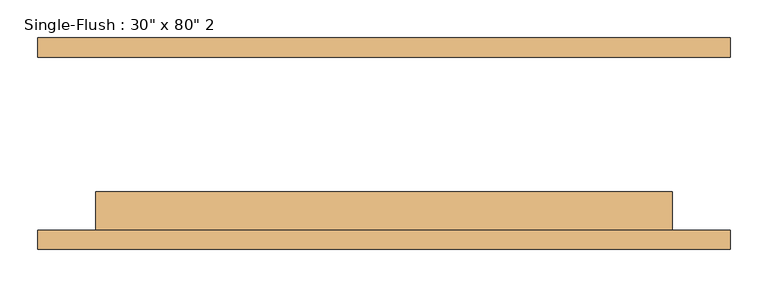
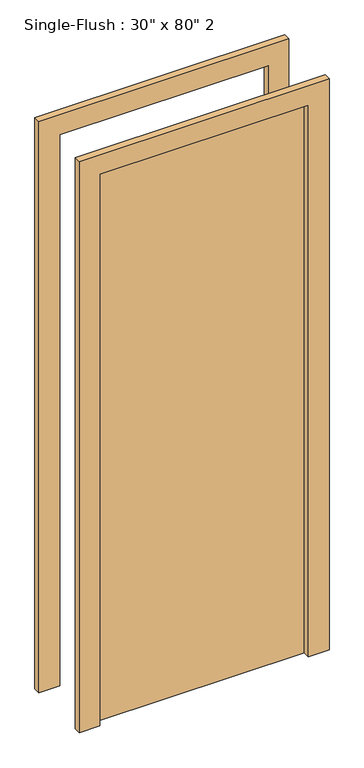
"""IFC4 building model written with IfcOpenShell, lengths in millimetres: door geometry."""

from ifc_helpers import new_model, si_unit, frame, origin, origin_with_axes, place, context, project, spatial, polyline, outline, extrude, source, transform, mapped, element, save


def door_5e1232af(model_context):
    return source(origin(), model_context, "Body", "SweptSolid", [
        extrude(outline(polyline([(2209.8, -457.2), (0.0, -457.2), (0.0, -381.0), (2133.6, -381.0), (2133.6, 381.0), (0.0, 381.0), (0.0, 457.2), (2209.8, 457.2), (2209.8, -457.2)])), frame((0.0, -139.7, 0.0), z_axis=(0.0, 1.0, 0.0), x_axis=(0.0, 0.0, 1.0)), (0.0, 0.0, 1.0), 25.4),
        extrude(outline(polyline([(2209.8, 457.2), (2209.8, -457.2), (0.0, -457.2), (0.0, -381.0), (2133.6, -381.0), (2133.6, 381.0), (0.0, 381.0), (0.0, 457.2), (2209.8, 457.2)])), frame((0.0, 114.3, 0.0), z_axis=(0.0, 1.0, 0.0), x_axis=(0.0, 0.0, 1.0)), (0.0, 0.0, 1.0), 25.4),
        extrude(outline(polyline([(381.0, -63.5), (381.0, -114.3), (-381.0, -114.3), (-381.0, -63.5), (381.0, -63.5)])), origin_with_axes(), (0.0, 0.0, 1.0), 2133.6),
    ])


if __name__ == "__main__":
    model = new_model("IFC4")
    model_context = context("Model", 3, world=origin())
    ifc_project = project(units=[si_unit("LENGTHUNIT", "METRE", prefix="MILLI")], contexts=[model_context])
    site = spatial("IfcSite", under=ifc_project)
    building = spatial("IfcBuilding", under=site)
    placement = place(None, origin())
    door_shape = door_5e1232af(model_context)
    element("IfcDoor", 1, ObjectType="Single-Flush : 30\" x 80\" 2", at=placement, inside=building, context=model_context, shape_type="MappedRepresentation", body=[
        mapped(door_shape, transform((0.0, 0.0, 0.0), x_axis=(1.0, 0.0, 0.0), y_axis=(0.0, 1.0, 0.0), z_axis=(0.0, 0.0, 1.0))),
    ])
    save(model, "model.ifc")

# Revit data of these elements
# Type "Single-Flush : 30\" x 80\" 2"
#   Type Mark = "14"
#   Construction Type Id = "MDOOR"
#   Assembly Code = "C1020"
#   Analytic Construction = "Metal"
#   Thickness = 0' - 2"
#   Heat Transfer Coefficient (U) = 0.651978 BTU/(h·ft²·°F)
#   Height = 7' - 0"
#   Trim Projection Ext = 0' - 1"
#   Trim Projection Int = 0' - 1"
#   Trim Width = 0' - 3"
#   Width = 2' - 6"
#   Define Thermal Properties by = 1
#   Door Material = Door - Panel
#   Frame Material = Door - Frame
#   Visual Light Transmittance = 0
#   Solar Heat Gain Coefficient = 0
#   Function = (empty or 0)
#   Wall Closure = (empty or 0)
# Element 1 (IfcDoor, "Single-Flush : 30\" x 80\" 2")
#   Materials on its faces: "Door - Frame", "Door - Panel"
# Materials
#   "Door - Panel": class "Wood", colour RGB 210 159 95, transparency 0, Cost = 0
#   "Door - Frame": colour RGB 118 70 51, transparency 0, Cost = 0
